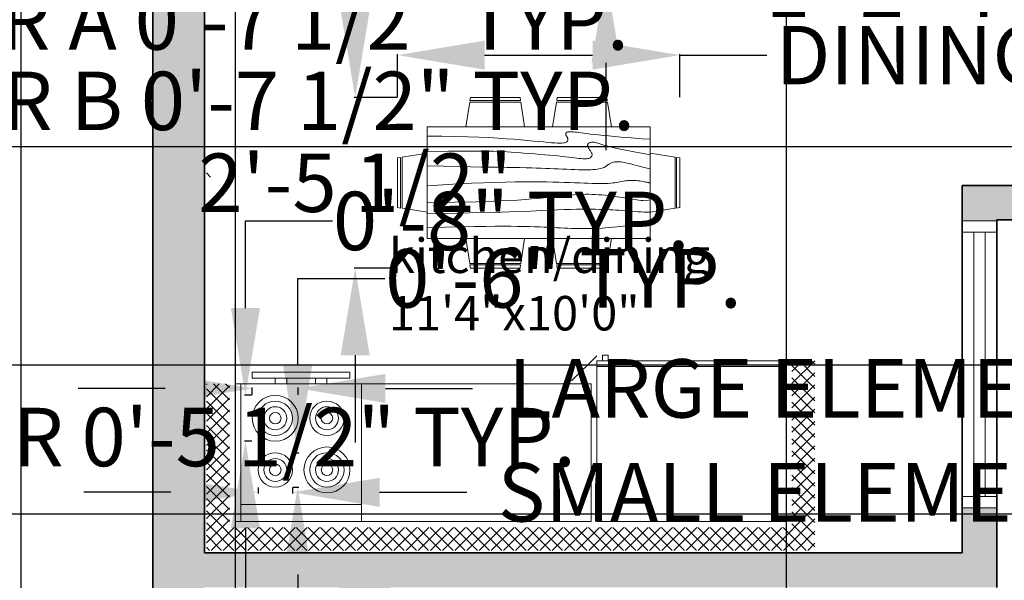
# Model space of a CAD drawing. Units: inches. Extents: x 19 to 15718, y 7 to 930.
# Tile 7 of 11: x 15243 to 15415, y 458 to 556. Entities that reach past the tile are written whole.
import ezdxf

# ---------------------------------------------------------------- set-up
doc = ezdxf.new("R2010")
doc.units = ezdxf.units.IN
doc.header["$MEASUREMENT"] = 0
for name, color, linetype, lineweight in [('A-ANNO-DIMS', 2, 'Continuous', 18), ('A-AREA-IDEN', 7, 'Continuous', 18), ('A-EQPM', 9, 'Continuous', 18), ('A-FLOR-CASE', 8, 'Continuous', 18), ('A-FLOR-CASE-PATT', 252, 'Continuous', 13), ('A-FURN', 8, 'Continuous', 18), ('A-GLAZ', 4, 'Continuous', 18), ('A-WALL', 7, 'Continuous', 35)]:
    doc.layers.add(name, color=color, linetype=linetype, lineweight=lineweight)
doc.layers.add('A-WALL-PATT', color=18, linetype='Continuous', lineweight=13, true_color=0x000000)
doc.styles.add('Annotative', font='arial.ttf')
doc.styles.get("Standard").update_dxf_attribs({"font": 'arial.ttf'})
doc.dimstyles.get("Standard").update_dxf_attribs({"dimtxt": 10.18, "dimasz": 15.18, "dimexe": 0.18, "dimexo": 0.0625, "dimgap": 0.09, "dimtad": 0, "dimtih": 1, "dimtoh": 1, "dimdec": 0, "dimzin": 0, "dimdsep": 46, "dimlunit": 3, "dimtxsty": 'Standard', "dimcen": 0.09, "dimadec": 0, "dimazin": 0, "dimtfac": 1, "dimtdec": 0, "dimtofl": 0, "dimtmove": 0, "dimatfit": 3, "dimfxl": 1, "dimtolj": 1, "dimtzin": 0, "dimarcsym": 0})

# ---------------------------------------------------------------- blocks, each defined once
blk = doc.blocks.new('Dining Set - 36 x 72 in.')
for p, q in [((-22.2343, 26.00059), (-23.4847, 17.99762)), ((-22.2304, 26), (-5.7608, 26)), ((-22, 27.5), (-22.1562, 26.50042)), ((-5.8416, 26.5), (-22.1534, 26.5)), ((-22, 27.5), (-6, 27.5)), ((-5.8437, 26.49966), (-6, 27.5)), ((-4.5152, 17.99762), (-5.7655, 25.99926)), ((5.7657, 26.00059), (4.5153, 17.99762)), ((5.7696, 26), (22.2392, 26)), ((6, 27.5), (5.8438, 26.50042)), ((22.1584, 26.5), (5.8466, 26.5)), ((6, 27.5), (22, 27.5)), ((22.1563, 26.49966), (22, 27.5)), ((23.4848, 17.99762), (22.2345, 25.99926)), ((36, 18), (-36, 18)), ((-36, 18), (-36, -18)), ((36, -18), (36, 18)), ((-45.5, 8), (-44.5004, 8.15617)), ((-45.5, 8), (-45.5, -8)), ((-44.5, -8.15843), (-44.5, 8.15338)), ((-44.0006, 8.23428), (-35.9976, 9.48474)), ((-44, 8.23041), (-44, -8.23915)), ((44.0006, 8.23428), (35.9976, 9.48474)), ((44, 8.23041), (44, -8.23915)), ((44.5, -8.15843), (44.5, 8.15338)), ((45.5, 8), (44.5005, 8.15617)), ((45.5, 8), (45.5, -8)), ((-44.4997, -8.15631), (-45.5, -8)), ((-35.9976, -9.48476), (-43.9993, -8.2345)), ((35.9976, -9.48476), (43.9993, -8.2345)), ((44.4997, -8.15631), (45.5, -8)), ((-36, -18), (36, -18)), ((-22.2343, -26.0006), (-23.4847, -17.99762)), ((-4.5152, -17.99762), (-5.7655, -25.99928)), ((5.7657, -26.0006), (4.5153, -17.99762)), ((23.4848, -17.99762), (22.2345, -25.99928)), ((-22.2304, -26), (-5.7608, -26)), ((-22, -27.5), (-22.1562, -26.50044)), ((-5.8416, -26.5), (-22.1534, -26.5)), ((-22, -27.5), (-6, -27.5)), ((-5.8437, -26.49967), (-6, -27.5)), ((5.7696, -26), (22.2392, -26)), ((6, -27.5), (5.8438, -26.50044)), ((22.1584, -26.5), (5.8466, -26.5)), ((6, -27.5), (22, -27.5)), ((22.1563, -26.49967), (22, -27.5))]:
    blk.add_line(p, q)
for points in [[(-36, 15), (-31.1772, 14.97754), (-26.8079, 14.91406), (-22.8538, 14.81543), (-19.276, 14.6875), (-16.0362, 14.53613), (-13.0957, 14.36718), (-10.4159, 14.18652), (-7.9583, 14), (-5.6904, 13.81315), (-3.6035, 13.63021), (-1.6954, 13.45508), (0.0365, 13.29166), (1.5945, 13.14388), (2.9811, 13.01562), (4.1988, 12.9108), (5.25, 12.83333), (6.1393, 12.78613), (6.8802, 12.76823), (7.4883, 12.77767), (7.9792, 12.8125), (8.3685, 12.87077), (8.6719, 12.95052), (8.9049, 13.0498), (9.0833, 13.16666), (9.2205, 13.29899), (9.3216, 13.44401), (9.3895, 13.59879), (9.4271, 13.76041), (9.4373, 13.92594), (9.4232, 14.09245), (9.3875, 14.257), (9.3333, 14.41666), (9.2638, 14.56917), (9.1836, 14.71484), (9.0975, 14.85465), (9.0104, 14.98958), (8.9272, 15.1206), (8.8529, 15.2487), (8.7922, 15.37483), (8.75, 15.5), (8.7305, 15.62467), (8.7344, 15.74739), (8.7617, 15.86621), (8.8125, 15.97916), (8.8867, 16.08431), (8.9844, 16.17968), (9.1055, 16.26334), (9.25, 16.33333), (9.4189, 16.38802), (9.6172, 16.42708), (9.8506, 16.45052), (10.125, 16.45833), (10.4463, 16.45052), (10.8203, 16.42708), (11.2529, 16.38802), (11.75, 16.33333), (12.3184, 16.26318), (12.9694, 16.17838), (13.7151, 16.07991), (14.5677, 15.96875), (15.5395, 15.84586), (16.6426, 15.71224), (17.8893, 15.56884), (19.2917, 15.41666), (20.859, 15.25667), (22.5879, 15.08984), (24.4721, 14.91715), (26.5052, 14.73958), (28.6809, 14.5581), (30.9929, 14.3737), (33.4347, 14.18733), (36, 14)], [(-36, 10), (-28.9766, 10.14274), (-23.1725, 10.20442), (-18.4241, 10.19775), (-14.5677, 10.13541), (-11.4399, 10.03011), (-8.877, 9.89453), (-6.7154, 9.74137), (-4.7917, 9.58333), (-2.9698, 9.43082), (-1.2246, 9.28515), (0.4415, 9.14534), (2.026, 9.01041), (3.5266, 8.87939), (4.9408, 8.7513), (6.266, 8.62516), (7.5, 8.5), (8.6411, 8.37549), (9.6914, 8.2539), (10.6538, 8.13818), (11.5312, 8.03125), (12.3267, 7.93603), (13.043, 7.85547), (13.6831, 7.79248), (14.25, 7.75), (14.7471, 7.7303), (15.1797, 7.73307), (15.5537, 7.75732), (15.875, 7.80208), (16.1494, 7.86637), (16.3828, 7.94922), (16.5811, 8.04964), (16.75, 8.16666), (16.8944, 8.29915), (17.0143, 8.44531), (17.1089, 8.60319), (17.1771, 8.77083), (17.218, 8.94629), (17.2305, 9.1276), (17.2137, 9.31282), (17.1667, 9.5), (17.0895, 9.6875), (16.987, 9.875), (16.8649, 10.0625), (16.7292, 10.25), (16.5856, 10.4375), (16.4401, 10.625), (16.2985, 10.8125), (16.1667, 11), (16.05, 11.18733), (15.9518, 11.3737), (15.8752, 11.5581), (15.8229, 11.73958), (15.798, 11.91715), (15.8034, 12.08984), (15.842, 12.25667), (15.9167, 12.41666), (16.0295, 12.56836), (16.1784, 12.70833), (16.3605, 12.83268), (16.5729, 12.9375), (16.8127, 13.01888), (17.0768, 13.07291), (17.3625, 13.0957), (17.6667, 13.08333), (17.9894, 13.03312), (18.3418, 12.94726), (18.7382, 12.82918), (19.1927, 12.68229), (19.7195, 12.51001), (20.3327, 12.31575), (21.0465, 12.10294), (21.875, 11.875), (22.8357, 11.63354), (23.959, 11.37304), (25.2786, 11.08618), (26.8282, 10.76562), (28.6414, 10.40405), (30.752, 9.99414), (33.1936, 9.52856), (36, 9)], [(-36, 5.5), (-30.7157, 5.3348), (-26.069, 5.20963), (-21.9946, 5.11767), (-18.4271, 5.05208), (-15.3009, 5.00602), (-12.5508, 4.97265), (-10.1112, 4.94515), (-7.9167, 4.91666), (-5.909, 4.88167), (-4.0586, 4.83984), (-2.3429, 4.79215), (-0.7396, 4.73958), (0.7739, 4.6831), (2.22, 4.6237), (3.6213, 4.56233), (5, 4.5), (6.373, 4.43782), (7.7344, 4.3776), (9.0723, 4.32129), (10.375, 4.27083), (11.6309, 4.22819), (12.8281, 4.19531), (13.9551, 4.17415), (15, 4.16666), (15.954, 4.17448), (16.819, 4.19791), (17.6001, 4.23698), (18.3021, 4.29166), (18.9299, 4.36198), (19.4883, 4.44791), (19.9823, 4.54948), (20.4167, 4.66666), (20.7969, 4.79899), (21.1302, 4.94401), (21.4245, 5.09879), (21.6875, 5.26041), (21.9271, 5.42594), (22.1511, 5.59245), (22.3672, 5.757), (22.5834, 5.91666), (22.8065, 6.06868), (23.0404, 6.21093), (23.2879, 6.34147), (23.5521, 6.45833), (23.8358, 6.55957), (24.142, 6.64323), (24.4735, 6.70735), (24.8334, 6.75), (25.2235, 6.76969), (25.642, 6.76692), (26.0858, 6.74267), (26.5521, 6.69791), (27.0379, 6.63362), (27.5404, 6.55078), (28.0565, 6.45036), (28.5834, 6.33333), (29.1242, 6.19987), (29.7071, 6.04687), (30.3661, 5.87044), (31.1354, 5.66666), (32.0493, 5.43164), (33.142, 5.16146), (34.4475, 4.85221), (36, 4.5)], [(-36, -1), (-30.7915, -0.6591), (-26.0195, -0.38216), (-21.6519, -0.16284), (-17.6563, 0.00521), (-14.0005, 0.12833), (-10.6523, 0.21289), (-7.5796, 0.26522), (-4.75, 0.29166), (-2.134, 0.29793), (0.2878, 0.28711), (2.5317, 0.26163), (4.6146, 0.22396), (6.5529, 0.17651), (8.3633, 0.12174), (10.0623, 0.06209), (11.6667, 0), (13.1899, -0.06201), (14.6341, -0.1211), (15.9982, -0.17432), (17.2813, -0.21875), (18.4823, -0.25147), (19.6003, -0.26953), (20.6343, -0.27002), (21.5834, -0.25), (22.4481, -0.20768), (23.2357, -0.14584), (23.9549, -0.06836), (24.6146, 0.02083), (25.2235, 0.11784), (25.7904, 0.21875), (26.3241, 0.31966), (26.8334, 0.41666), (27.3265, 0.50618), (27.8099, 0.58593), (28.2894, 0.65397), (28.7709, 0.70833), (29.2601, 0.74707), (29.763, 0.76823), (30.2855, 0.76985), (30.8334, 0.75), (31.4088, 0.70784), (31.9994, 0.64713), (32.589, 0.57275), (33.1615, 0.48958), (33.7008, 0.4025), (34.1908, 0.3164), (34.6153, 0.23616), (34.9584, 0.16666), (35.2099, 0.11165), (35.3848, 0.07031), (35.504, 0.04069), (35.5886, 0.02083), (35.6594, 0.00879), (35.7377, 0.0026), (35.8442, 0.00032), (36, 0)], [(-36, -6.5), (-27.1843, -6.31267), (-20.084, -6.1263), (-14.469, -5.9419), (-10.1094, -5.76042), (-6.7752, -5.58285), (-4.2363, -5.41016), (-2.2629, -5.24333), (-0.625, -5.08334), (0.8708, -4.93099), (2.2715, -4.78646), (3.5872, -4.64974), (4.8281, -4.52084), (6.0046, -4.39974), (7.127, -4.28646), (8.2053, -4.18099), (9.25, -4.08334), (10.2705, -3.99382), (11.2734, -3.91407), (12.2647, -3.84603), (13.25, -3.79167), (14.2354, -3.75293), (15.2266, -3.73177), (16.2295, -3.73015), (17.25, -3.75), (18.2912, -3.79248), (19.3451, -3.85547), (20.4009, -3.93604), (21.4479, -4.03125), (22.4754, -4.13819), (23.4727, -4.25391), (24.4289, -4.37549), (25.3334, -4.5), (26.1785, -4.62492), (26.9694, -4.74935), (27.7145, -4.87281), (28.4219, -4.99479), (29.1, -5.11483), (29.7572, -5.23242), (30.4016, -5.34709), (31.0417, -5.45834), (31.6837, -5.56437), (32.3262, -5.65821), (32.9658, -5.73153), (33.599, -5.77604), (34.2224, -5.78345), (34.8327, -5.74545), (35.4264, -5.65373), (36, -5.5)], [(-36, -10), (-26.4022, -9.81299), (-18.4675, -9.62891), (-11.9839, -9.45069), (-6.7396, -9.28125), (-2.5226, -9.12354), (0.8789, -8.98047), (3.6769, -8.85498), (6.0833, -8.75), (8.2767, -8.66765), (10.3021, -8.60677), (12.1712, -8.56543), (13.8958, -8.54167), (15.4876, -8.53353), (16.9583, -8.53907), (18.3197, -8.55632), (19.5834, -8.58334), (20.7616, -8.61841), (21.8685, -8.66081), (22.9188, -8.71004), (23.9271, -8.76563), (24.9081, -8.82707), (25.8763, -8.89388), (26.8465, -8.96558), (27.8334, -9.04167), (28.8474, -9.12118), (29.8828, -9.20117), (30.93, -9.27824), (31.9792, -9.34896), (33.0205, -9.40991), (34.0443, -9.45768), (35.0407, -9.48885), (36, -9.5)], [(-36, -14.5), (-30.0881, -14.33513), (-25.0332, -14.21224), (-20.7312, -14.12647), (-17.0781, -14.07292), (-13.97, -14.04671), (-11.3027, -14.04297), (-8.9724, -14.05681), (-6.875, -14.08334), (-4.9224, -14.11833), (-3.0905, -14.16016), (-1.3709, -14.20785), (0.2448, -14.26042), (1.7647, -14.3169), (3.1973, -14.3763), (4.5507, -14.43767), (5.8333, -14.5), (7.0554, -14.5621), (8.235, -14.62175), (9.3922, -14.67652), (10.5469, -14.72396), (11.7192, -14.76164), (12.929, -14.78711), (14.1965, -14.79794), (15.5417, -14.79167), (16.9933, -14.76424), (18.6152, -14.70508), (20.4804, -14.60197), (22.6615, -14.44271), (25.2312, -14.21509), (28.2624, -13.9069), (31.8277, -13.50594), (36, -13)]]:
    blk.add_lwpolyline(points)
blk = doc.blocks.new('*D17')
at = {"layer": 'A-ANNO-DIMS', "color": 0, "lineweight": -2, "transparency": 16777216}
for p, q in [((15266.62, 830.27), (15243.58, 830.27)), ((15243.76, 815.09), (15243.76, 595.52)), ((15243.76, 365.38), (15243.76, 584.95)), ((15266.62, 350.2), (15243.58, 350.2))]:
    blk.add_line(p, q, dxfattribs=at)
at = {"layer": 'A-ANNO-DIMS', "color": 0, "transparency": 16777216}
for points in [[(15241.23, 815.09), (15246.29, 815.09), (15243.76, 830.27)], [(15241.23, 365.38), (15246.29, 365.38), (15243.76, 350.2)]]:
    blk.add_solid(points, dxfattribs=at)
at = {"layer": 'Defpoints', "color": 0, "transparency": 16777216}
for p in [(15266.68, 830.27), (15243.76, 350.2), (15266.68, 350.2)]:
    blk.add_point(p, dxfattribs=at)
at = {"layer": 'A-ANNO-DIMS', "color": 0, "transparency": 16777216, "insert": (15243.76, 590.24), "char_height": 10.18, "attachment_point": 5}
blk.add_mtext("\\A1;40'", dxfattribs=at)
blk = doc.blocks.new('HOB-ELECTRIC-6IN')
for radius in [3, 2, 1]:
    blk.add_circle((3, 3), radius)
blk = doc.blocks.new('HOB-ELECTRIC-8IN')
for radius in [4, 3, 2, 1]:
    blk.add_circle((4, 4), radius)
blk = doc.blocks.new('*D40')
at = {"layer": 'A-ANNO-DIMS', "color": 0, "lineweight": -2, "transparency": 16777216}
for p, q in [((15117.25, 555.92), (15102.07, 555.92)), ((15132.43, 556.96), (15132.43, 555.74)), ((15139.78, 556.96), (15139.78, 555.74)), ((15154.96, 555.92), (15170.14, 555.92))]:
    blk.add_line(p, q, dxfattribs=at)
at = {"layer": 'A-ANNO-DIMS', "color": 0, "transparency": 16777216}
for points in [[(15117.25, 558.45), (15117.25, 553.39), (15132.43, 555.92)], [(15154.96, 558.45), (15154.96, 553.39), (15139.78, 555.92)]]:
    blk.add_solid(points, dxfattribs=at)
at = {"layer": 'Defpoints', "color": 0, "transparency": 16777216}
for p in [(15132.43, 557.02), (15139.78, 557.02), (15139.78, 555.92)]:
    blk.add_point(p, dxfattribs=at)
at = {"layer": 'A-ANNO-DIMS', "color": 0, "transparency": 16777216, "insert": (15262.49, 555.92), "char_height": 10.18, "attachment_point": 5}
blk.add_mtext('\\A1;SIDE CHAIR A 0\'-7 1/2" TYP.', dxfattribs=at)
blk = doc.blocks.new('*D42')
at = {"layer": 'A-ANNO-DIMS', "color": 0, "lineweight": -2, "transparency": 16777216}
for p, q in [((15133.17, 540.88), (15133.17, 542.1)), ((15140.52, 540.88), (15140.52, 542.1)), ((15117.99, 541.92), (15102.81, 541.92)), ((15155.7, 541.92), (15170.88, 541.92))]:
    blk.add_line(p, q, dxfattribs=at)
at = {"layer": 'A-ANNO-DIMS', "color": 0, "transparency": 16777216}
for points in [[(15117.99, 544.45), (15117.99, 539.39), (15133.17, 541.92)], [(15155.7, 544.45), (15155.7, 539.39), (15140.52, 541.92)]]:
    blk.add_solid(points, dxfattribs=at)
at = {"layer": 'Defpoints', "color": 0, "transparency": 16777216}
for p in [(15133.17, 540.82), (15140.52, 541.92), (15140.52, 540.82)]:
    blk.add_point(p, dxfattribs=at)
at = {"layer": 'A-ANNO-DIMS', "color": 0, "transparency": 16777216, "insert": (15263.22, 541.92), "char_height": 10.18, "attachment_point": 5}
blk.add_mtext('\\A1;SIDE CHAIR B 0\'-7 1/2" TYP.', dxfattribs=at)
blk = doc.blocks.new('*D60')
at = {"layer": 'A-ANNO-DIMS', "color": 0, "lineweight": -2, "transparency": 16777216}
for p, q in [((15125.78, 484.16), (15125.78, 483.21)), ((15131.32, 484.16), (15131.32, 483.21)), ((15110.6, 483.39), (15095.42, 483.39)), ((15146.5, 483.39), (15161.68, 483.39))]:
    blk.add_line(p, q, dxfattribs=at)
at = {"layer": 'A-ANNO-DIMS', "color": 0, "transparency": 16777216}
for points in [[(15110.6, 485.92), (15110.6, 480.86), (15125.78, 483.39)], [(15146.5, 485.92), (15146.5, 480.86), (15131.32, 483.39)]]:
    blk.add_solid(points, dxfattribs=at)
at = {"layer": 'Defpoints', "color": 0, "transparency": 16777216}
for p in [(15125.78, 484.23), (15131.32, 484.23), (15131.32, 483.39)]:
    blk.add_point(p, dxfattribs=at)
at = {"layer": 'A-ANNO-DIMS', "color": 0, "transparency": 16777216, "insert": (15253.56, 483.39), "char_height": 10.18, "attachment_point": 5}
blk.add_mtext('\\A1;GAS BURNER 0\'-5 1/2" TYP.', dxfattribs=at)
blk = doc.blocks.new('*D62')
at = {"layer": 'A-ANNO-DIMS', "color": 0, "lineweight": -2, "transparency": 16777216}
for p, q in [((15269.83, 473.76), (15254.65, 473.76)), ((15285.01, 474.6), (15285.01, 473.58)), ((15291.01, 474.6), (15291.01, 473.58)), ((15306.19, 473.76), (15321.37, 473.76))]:
    blk.add_line(p, q, dxfattribs=at)
at = {"layer": 'A-ANNO-DIMS', "color": 0, "transparency": 16777216}
for points in [[(15269.83, 476.29), (15269.83, 471.23), (15285.01, 473.76)], [(15306.19, 476.29), (15306.19, 471.23), (15291.01, 473.76)]]:
    blk.add_solid(points, dxfattribs=at)
at = {"layer": 'Defpoints', "color": 0, "transparency": 16777216}
for p in [(15285.01, 474.66), (15291.01, 474.66), (15291.01, 473.76)]:
    blk.add_point(p, dxfattribs=at)
at = {"layer": 'A-ANNO-DIMS', "color": 0, "transparency": 16777216, "insert": (15413.32, 473.76), "char_height": 10.18, "attachment_point": 5}
blk.add_mtext('\\A1;SMALL ELEMENT 0\'-6" TYP.', dxfattribs=at)
blk = doc.blocks.new('*D63')
at = {"layer": 'A-ANNO-DIMS', "color": 0, "lineweight": -2, "transparency": 16777216}
for p, q in [((15291.91, 495.84), (15291.91, 511.02)), ((15291.91, 511.02), (15307.09, 511.02)), ((15291.07, 480.66), (15292.09, 480.66)), ((15291.07, 474.66), (15292.09, 474.66)), ((15291.91, 459.48), (15291.91, 444.3))]:
    blk.add_line(p, q, dxfattribs=at)
at = {"layer": 'A-ANNO-DIMS', "color": 0, "transparency": 16777216}
for points in [[(15289.38, 495.84), (15294.44, 495.84), (15291.91, 480.66)], [(15289.38, 459.48), (15294.44, 459.48), (15291.91, 474.66)]]:
    blk.add_solid(points, dxfattribs=at)
at = {"layer": 'Defpoints', "color": 0, "transparency": 16777216}
for p in [(15291.01, 480.66), (15291.91, 480.66), (15291.01, 474.66)]:
    blk.add_point(p, dxfattribs=at)
at = {"layer": 'A-ANNO-DIMS', "color": 0, "transparency": 16777216, "insert": (15338.21, 511.02), "char_height": 10.18, "attachment_point": 5}
blk.add_mtext('\\A1;0\'-6" TYP.', dxfattribs=at)
blk = doc.blocks.new('*D64')
at = {"layer": 'A-ANNO-DIMS', "color": 0, "lineweight": -2, "transparency": 16777216}
for p, q in [((15268.83, 491.86), (15253.65, 491.86)), ((15284.01, 490.72), (15284.01, 492.04)), ((15292.01, 490.72), (15292.01, 492.04)), ((15307.19, 491.86), (15322.37, 491.86))]:
    blk.add_line(p, q, dxfattribs=at)
at = {"layer": 'A-ANNO-DIMS', "color": 0, "transparency": 16777216}
for points in [[(15268.83, 494.39), (15268.83, 489.33), (15284.01, 491.86)], [(15307.19, 494.39), (15307.19, 489.33), (15292.01, 491.86)]]:
    blk.add_solid(points, dxfattribs=at)
at = {"layer": 'Defpoints', "color": 0, "transparency": 16777216}
for p in [(15284.01, 490.66), (15292.01, 491.86), (15292.01, 490.66)]:
    blk.add_point(p, dxfattribs=at)
at = {"layer": 'A-ANNO-DIMS', "color": 0, "transparency": 16777216, "insert": (15414.9, 491.86), "char_height": 10.18, "attachment_point": 5}
blk.add_mtext('\\A1;LARGE ELEMENT 0\'-8" TYP.', dxfattribs=at)
blk = doc.blocks.new('*D65')
at = {"layer": 'A-ANNO-DIMS', "color": 0, "lineweight": -2, "transparency": 16777216}
for p, q in [((15282.81, 505.84), (15282.81, 521.02)), ((15282.81, 521.02), (15297.99, 521.02)), ((15283.95, 490.66), (15282.63, 490.66)), ((15283.95, 482.66), (15282.63, 482.66)), ((15282.81, 467.48), (15282.81, 452.3))]:
    blk.add_line(p, q, dxfattribs=at)
at = {"layer": 'A-ANNO-DIMS', "color": 0, "transparency": 16777216}
for points in [[(15280.28, 505.84), (15285.34, 505.84), (15282.81, 490.66)], [(15280.28, 467.48), (15285.34, 467.48), (15282.81, 482.66)]]:
    blk.add_solid(points, dxfattribs=at)
at = {"layer": 'Defpoints', "color": 0, "transparency": 16777216}
for p in [(15282.81, 490.66), (15284.01, 490.66), (15284.01, 482.66)]:
    blk.add_point(p, dxfattribs=at)
at = {"layer": 'A-ANNO-DIMS', "color": 0, "transparency": 16777216, "insert": (15329.11, 521.02), "char_height": 10.18, "attachment_point": 5}
blk.add_mtext('\\A1;0\'-8" TYP.', dxfattribs=at)
blk = doc.blocks.new('*D66')
at = {"layer": 'A-ANNO-DIMS', "color": 0, "lineweight": -2, "transparency": 16777216}
for p, q in [((15345.61, 592.88), (15345.61, 608.06)), ((15343.57, 577.7), (15345.79, 577.7)), ((15343.57, 563.7), (15345.79, 563.7)), ((15345.61, 548.52), (15345.61, 533.34))]:
    blk.add_line(p, q, dxfattribs=at)
at = {"layer": 'A-ANNO-DIMS', "color": 0, "transparency": 16777216}
for points in [[(15343.08, 592.88), (15348.14, 592.88), (15345.61, 577.7)], [(15343.08, 548.52), (15348.14, 548.52), (15345.61, 563.7)]]:
    blk.add_solid(points, dxfattribs=at)
at = {"layer": 'Defpoints', "color": 0, "transparency": 16777216}
for p in [(15343.51, 577.7), (15345.61, 577.7), (15343.51, 563.7)]:
    blk.add_point(p, dxfattribs=at)
at = {"layer": 'A-ANNO-DIMS', "color": 0, "transparency": 16777216, "insert": (15345.61, 570.7), "char_height": 10.18, "attachment_point": 5}
blk.add_mtext('\\A1;SINK BOWL 1\'-2" TYP.', dxfattribs=at)
blk = doc.blocks.new('*D67')
at = {"layer": 'A-ANNO-DIMS', "color": 0, "lineweight": -2, "transparency": 16777216}
for p, q in [((15329.76, 563.64), (15329.76, 561.42)), ((15343.51, 563.64), (15343.51, 561.42)), ((15314.58, 561.6), (15299.4, 561.6)), ((15358.69, 561.6), (15373.87, 561.6))]:
    blk.add_line(p, q, dxfattribs=at)
at = {"layer": 'A-ANNO-DIMS', "color": 0, "transparency": 16777216}
for points in [[(15314.58, 564.13), (15314.58, 559.07), (15329.76, 561.6)], [(15358.69, 564.13), (15358.69, 559.07), (15343.51, 561.6)]]:
    blk.add_solid(points, dxfattribs=at)
at = {"layer": 'Defpoints', "color": 0, "transparency": 16777216}
for p in [(15329.76, 563.7), (15343.51, 563.7), (15343.51, 561.6)]:
    blk.add_point(p, dxfattribs=at)
at = {"layer": 'A-ANNO-DIMS', "color": 0, "transparency": 16777216, "insert": (15404.51, 561.6), "char_height": 10.18, "attachment_point": 5}
blk.add_mtext('\\A1;1\'-2" TYP.', dxfattribs=at)
blk = doc.blocks.new('*D68')
at = {"layer": 'A-ANNO-DIMS', "color": 0, "lineweight": -2, "transparency": 16777216}
for p, q in [((15309.3, 542.58), (15309.3, 550.07)), ((15324.48, 549.89), (15343.27, 549.89)), ((15358.45, 542.58), (15358.45, 550.07)), ((15358.45, 549.89), (15373.63, 549.89))]:
    blk.add_line(p, q, dxfattribs=at)
at = {"layer": 'A-ANNO-DIMS', "color": 0, "transparency": 16777216}
for points in [[(15324.48, 552.42), (15324.48, 547.36), (15309.3, 549.89)], [(15343.27, 552.42), (15343.27, 547.36), (15358.45, 549.89)]]:
    blk.add_solid(points, dxfattribs=at)
at = {"layer": 'Defpoints', "color": 0, "transparency": 16777216}
for p in [(15358.45, 549.89), (15309.3, 542.52), (15358.45, 542.52)]:
    blk.add_point(p, dxfattribs=at)
at = {"layer": 'A-ANNO-DIMS', "color": 0, "transparency": 16777216, "insert": (15429.66, 549.89), "char_height": 10.18, "attachment_point": 5}
blk.add_mtext('\\A1;DINING SET 4\'-1"', dxfattribs=at)
blk = doc.blocks.new('*D69')
at = {"layer": 'A-ANNO-DIMS', "color": 0, "lineweight": -2, "transparency": 16777216}
for p, q in [((15301.93, 557.7), (15301.93, 572.88)), ((15309.24, 542.52), (15301.75, 542.52)), ((15309.24, 512.82), (15301.75, 512.82)), ((15301.93, 497.64), (15301.93, 482.46))]:
    blk.add_line(p, q, dxfattribs=at)
at = {"layer": 'A-ANNO-DIMS', "color": 0, "transparency": 16777216}
for points in [[(15299.4, 557.7), (15304.46, 557.7), (15301.93, 542.52)], [(15299.4, 497.64), (15304.46, 497.64), (15301.93, 512.82)]]:
    blk.add_solid(points, dxfattribs=at)
at = {"layer": 'Defpoints', "color": 0, "transparency": 16777216}
for p in [(15301.93, 542.52), (15309.3, 542.52), (15309.3, 512.82)]:
    blk.add_point(p, dxfattribs=at)
at = {"layer": 'A-ANNO-DIMS', "color": 0, "transparency": 16777216, "insert": (15301.93, 527.67), "char_height": 10.18, "attachment_point": 5}
blk.add_mtext('\\A1;2\'-5 1/2"', dxfattribs=at)
blk = doc.blocks.new('*D79')
at = {"layer": 'A-ANNO-DIMS', "color": 0, "lineweight": -2, "transparency": 16777216}
for p, q in [((15602.03, 534), (15602.03, 549.18)), ((15602.03, 549.18), (15617.21, 549.18)), ((15082.89, 534), (15602.21, 534)), ((15602.03, 511.14), (15602.03, 518.82)), ((15082.89, 495.96), (15602.21, 495.96))]:
    blk.add_line(p, q, dxfattribs=at)
at = {"layer": 'A-ANNO-DIMS', "color": 0, "transparency": 16777216}
for points in [[(15599.5, 518.82), (15604.56, 518.82), (15602.03, 534)], [(15599.5, 511.14), (15604.56, 511.14), (15602.03, 495.96)]]:
    blk.add_solid(points, dxfattribs=at)
at = {"layer": 'Defpoints', "color": 0, "transparency": 16777216}
for p in [(15082.83, 534), (15602.03, 534), (15082.83, 495.96)]:
    blk.add_point(p, dxfattribs=at)
at = {"layer": 'A-ANNO-DIMS', "color": 0, "transparency": 16777216, "insert": (15630.83, 549.18), "char_height": 10.18, "attachment_point": 5}
blk.add_mtext('\\A1;3\'-2"', dxfattribs=at)
blk = doc.blocks.new('*D80')
at = {"layer": 'A-ANNO-DIMS', "color": 0, "lineweight": -2, "transparency": 16777216}
for p, q in [((15602.030581, 511.142303), (15602.030581, 526.322303)), ((15181.899116, 495.962303), (15602.210581, 495.962303)), ((15181.899116, 469.995573), (15602.210581, 469.995573)), ((15602.030581, 454.815573), (15602.030581, 439.635573))]:
    blk.add_line(p, q, dxfattribs=at)
at = {"layer": 'A-ANNO-DIMS', "color": 0, "transparency": 16777216}
for points in [[(15599.500581, 511.142303), (15604.560581, 511.142303), (15602.030581, 495.962303)], [(15599.500581, 454.815573), (15604.560581, 454.815573), (15602.030581, 469.995573)]]:
    blk.add_solid(points, dxfattribs=at)
at = {"layer": 'Defpoints', "color": 0, "transparency": 16777216}
for p in [(15181.836616, 495.962303), (15602.030581, 495.962303), (15181.836616, 469.995573)]:
    blk.add_point(p, dxfattribs=at)
at = {"layer": 'A-ANNO-DIMS', "color": 0, "transparency": 16777216, "insert": (15602.030581, 482.978938), "char_height": 10.18, "attachment_point": 5}
blk.add_mtext('\\A1;2\'-2"', dxfattribs=at)
blk = doc.blocks.new('*D81')
at = {"layer": 'A-ANNO-DIMS', "color": 0, "lineweight": -2, "transparency": 16777216}
for p, q in [((15281.01, 559.14), (15281.01, 314.67)), ((15377.01, 559.14), (15377.01, 314.67)), ((15296.19, 314.85), (15315.38, 314.85)), ((15361.83, 314.85), (15342.64, 314.85))]:
    blk.add_line(p, q, dxfattribs=at)
at = {"layer": 'A-ANNO-DIMS', "color": 0, "transparency": 16777216}
for points in [[(15296.19, 317.38), (15296.19, 312.32), (15281.01, 314.85)], [(15361.83, 317.38), (15361.83, 312.32), (15377.01, 314.85)]]:
    blk.add_solid(points, dxfattribs=at)
at = {"layer": 'Defpoints', "color": 0, "transparency": 16777216}
for p in [(15281.01, 559.2), (15377.01, 559.2), (15377.01, 314.85)]:
    blk.add_point(p, dxfattribs=at)
at = {"layer": 'A-ANNO-DIMS', "color": 0, "transparency": 16777216, "insert": (15329.01, 314.85), "char_height": 10.18, "attachment_point": 5}
blk.add_mtext('\\A1;8\'-0"', dxfattribs=at)
blk = doc.blocks.new('*D82')
at = {"layer": 'A-ANNO-DIMS', "color": 0, "lineweight": -2, "transparency": 16777216}
for p, q in [((15602.030581, 598.383955), (15602.030581, 613.563955)), ((15377.073779, 583.203955), (15602.210581, 583.203955)), ((15377.073779, 559.203955), (15602.210581, 559.203955)), ((15602.030581, 544.023955), (15602.030581, 528.843955))]:
    blk.add_line(p, q, dxfattribs=at)
at = {"layer": 'A-ANNO-DIMS', "color": 0, "transparency": 16777216}
for points in [[(15599.500581, 598.383955), (15604.560581, 598.383955), (15602.030581, 583.203955)], [(15599.500581, 544.023955), (15604.560581, 544.023955), (15602.030581, 559.203955)]]:
    blk.add_solid(points, dxfattribs=at)
at = {"layer": 'Defpoints', "color": 0, "transparency": 16777216}
for p in [(15377.011279, 583.203955), (15602.030581, 583.203955), (15377.011279, 559.203955)]:
    blk.add_point(p, dxfattribs=at)
at = {"layer": 'A-ANNO-DIMS', "color": 0, "transparency": 16777216, "insert": (15602.030581, 571.203955), "char_height": 10.18, "attachment_point": 5}
blk.add_mtext('\\A1;2\'-0"', dxfattribs=at)

msp = doc.modelspace()

# ---------------------------------------------------------------- hatches: boundary and pattern name
at = {"layer": 'A-FLOR-CASE-PATT'}
h = msp.add_hatch(dxfattribs=at)
h.set_pattern_fill('ANSI37', color=256, scale=12, style=0)
h.paths.add_polyline_path([(15276.01, 463.66), (15382.01, 463.66), (15382.01, 496.66), (15378.01, 496.66), (15378.01, 467.66), (15280.01, 467.66), (15280.01, 492.66), (15276.01, 492.66)])
at = {"layer": 'A-WALL-PATT'}
h = msp.add_hatch(color=256, dxfattribs=at)
h.dxf.hatch_style = 1
h.paths.add_polyline_path([(15190.84, 837), (14890.84, 837), (14890.84, 357), (14899.84, 357), (14899.84, 366), (14899.84, 528), (14904.84, 528), (14904.84, 534), (14899.84, 534), (14899.84, 698), (15004.84, 698), (15004.84, 701, -0.014283), (15004.84, 703), (15004.84, 704), (14899.84, 704), (14899.84, 828), (14987.26, 828), (15043.84, 828), (15049.84, 828), (15075.84, 828), (15081.84, 828), (15181.84, 828), (15181.84, 780), (15114.84, 780), (15114.84, 779, -0.017236), (15114.84, 777), (15114.84, 774), (15181.84, 774), (15181.84, 654), (15181.84, 648), (15181.84, 596), (15190.84, 596)])
h.paths.add_polyline_path([(15190.84, 590), (15181.84, 590), (15181.84, 470), (15181.84, 464), (15181.84, 361.43), (14991.9, 361.43), (14991.5, 357), (15190.84, 357)], flags=0)
h.paths.add_polyline_path([(15152.29, 608), (15146.29, 608), (15146.29, 596), (15049.84, 596), (15049.84, 590), (15152.29, 590)], flags=17)
h.paths.add_polyline_path([(15049.84, 615), (15048.84, 615, -0.017236), (15046.84, 615), (15043.84, 615), (15043.84, 596), (15049.84, 596)], flags=17)
edge = h.paths.add_edge_path(flags=17)
edge.add_line((15152.29, 654), (15049.84, 654))
edge.add_line((15049.84, 654), (15043.84, 654))
edge.add_line((15043.84, 654), (15043.84, 648))
edge.add_line((15043.84, 648), (15049.84, 648))
edge.add_line((15049.84, 648), (15075.84, 648))
edge.add_line((15075.84, 648), (15081.84, 648))
edge.add_line((15081.84, 648), (15117.26, 648))
edge.add_spline(control_points=[(15117.26, 648), (15117.59, 648.02), (15117.94, 648.03), (15118.71, 648.04), (15119.15, 648.02), (15119.59, 648)], knot_values=[1.499122, 1.499122, 1.499122, 1.499122, 1.618335, 1.618335, 1.770388, 1.770388, 1.770388, 1.770388], degree=3, periodic=0)
edge.add_spline(control_points=[(15127.99, 642.93), (15128, 643.28), (15127.95, 643.62), (15127.73, 644.26), (15127.57, 644.57), (15127.16, 645.13), (15126.92, 645.39), (15126.04, 646.16), (15125.28, 646.6), (15123.53, 647.31), (15122.55, 647.59), (15120.88, 647.88), (15120.24, 647.95), (15119.59, 648)], knot_values=[0, 0, 0, 0, 0.172075, 0.172075, 0.344149, 0.344149, 0.516224, 0.516224, 0.894541, 0.894541, 1.272858, 1.272858, 1.499122, 1.499122, 1.499122, 1.499122], degree=3, periodic=0)
edge.add_line((15119.59, 648), (15146.29, 648))
edge.add_line((15146.29, 648), (15146.29, 636))
edge.add_line((15146.29, 636), (15152.29, 636))
edge.add_line((15152.29, 636), (15152.29, 654))
h.paths.add_polyline_path([(15132.35, 430.4), (15123.35, 430.4), (15123.35, 396.8), (15027.77, 396.8), (15027.77, 387.8), (15132.35, 387.8)], flags=17)
h.paths.add_polyline_path([(15132.35, 464), (15123.35, 464), (15123.35, 430.4), (15132.35, 430.4)], flags=17)
h.paths.add_polyline_path([(15275.68, 583.59), (15276.07, 583.2), (15276.65, 583.2), (15280.6, 587.16), (15278.55, 589.2), (15275.68, 589.2), (15275.68, 601.2), (15266.68, 601.2), (15266.68, 350.2), (15275.68, 350.2), (15275.68, 359.2), (15275.68, 457.2), (15413.68, 457.2), (15413.68, 471.04), (15407.68, 471.04), (15407.68, 463.2), (15275.68, 463.2)])
h = msp.add_hatch(color=256, dxfattribs=at)
h.dxf.hatch_style = 1
h.paths.add_polyline_path([(15566.68, 830.2), (15266.68, 830.2), (15266.68, 629.2), (15275.68, 629.2), (15275.68, 641.2), (15301.68, 641.2), (15301.68, 589.2), (15275.68, 589.2), (15275.68, 601.2), (15266.68, 601.2), (15266.68, 350.2), (15275.68, 350.2), (15275.68, 359.2), (15275.68, 457.2), (15413.68, 457.2), (15413.68, 471.04), (15407.68, 471.04), (15407.68, 463.2), (15275.68, 463.2), (15275.68, 583.59), (15276.07, 583.2), (15276.65, 583.2), (15277.42, 583.97), (15276.36, 585.03), (15279.54, 588.22), (15280.6, 587.16), (15281.66, 588.22), (15282.72, 587.16), (15283.78, 588.22), (15284.85, 587.16), (15285.91, 588.22), (15286.97, 587.16), (15288.03, 588.22), (15289.09, 587.16), (15290.15, 588.22), (15291.21, 587.16), (15292.27, 588.22), (15293.33, 587.16), (15294.39, 588.22), (15295.45, 587.16), (15296.51, 588.22), (15297.57, 587.16), (15298.63, 588.22), (15299.69, 587.16), (15300.76, 588.22), (15301.82, 587.16), (15302.88, 588.22), (15303.94, 587.16), (15305, 588.22), (15306.06, 587.16), (15307.68, 588.78), (15307.68, 641.2), (15407.68, 641.2), (15413.68, 641.2), (15413.68, 647.2), (15407.68, 647.2), (15275.68, 647.2), (15275.68, 767.2), (15336.68, 767.2), (15336.68, 773.2), (15275.68, 773.2), (15275.68, 821.2), (15375.68, 821.2), (15381.68, 821.2), (15407.68, 821.2), (15413.68, 821.2), (15557.68, 821.2), (15557.68, 697.2), (15452.68, 697.2), (15452.68, 696.2, -0.014283), (15452.68, 694.2), (15452.68, 691.2), (15557.68, 691.2), (15557.68, 527.2), (15557.68, 521.2), (15557.68, 359.2), (15557.68, 350.2), (15566.68, 350.2)])
h.paths.add_polyline_path([(15416.63, 527.2), (15413.68, 527.2), (15407.68, 527.2), (15407.68, 521.04), (15413.68, 521.04), (15413.68, 521.2), (15416.63, 521.2)], flags=17)
h.paths.add_polyline_path([(15432.13, 393.97), (15308.13, 393.97), (15308.13, 425.59), (15299.13, 425.59), (15299.13, 384.97), (15432.13, 384.97)], flags=17)
h.paths.add_polyline_path([(15308.13, 457.2), (15299.13, 457.2), (15299.13, 425.59), (15308.13, 425.59)], flags=17)
h.paths.add_polyline_path([(15425.57, 359.2), (15275.68, 359.2), (15275.68, 350.2), (15425.57, 350.2)], flags=17)
h.paths.add_polyline_path([(15413.68, 797.2), (15407.68, 797.2), (15407.68, 773.2), (15381.68, 773.2), (15381.68, 797.2), (15375.68, 797.2), (15375.68, 773.2), (15375.68, 767.2), (15407.68, 767.2), (15407.68, 686.2), (15408.68, 686.2, -0.014283), (15410.68, 686.2), (15413.68, 686.2), (15413.68, 691.2), (15413.68, 697.2)], flags=17)
h.paths.add_polyline_path([(15413.68, 608.2), (15410.68, 608.2, -0.017236), (15408.68, 608.2), (15407.68, 608.2), (15407.68, 589.2), (15388.16, 589.2, -0.313626), (15386.75, 588.23), (15381.37, 588.23), (15380.3, 587.16), (15381.37, 586.1), (15380.3, 585.03), (15382.14, 583.2), (15407.68, 583.2), (15413.68, 583.2)], flags=17)

# ---------------------------------------------------------------- linework, layer by layer
at = {"layer": 'A-EQPM'}
for p, q in [((15345.01, 497.66), (15346.01, 497.66)), ((15345.01, 496.66), (15345.01, 497.66)), ((15346.01, 497.66), (15346.01, 496.66)), ((15377.01, 495.66), (15344.01, 495.66)), ((15288.01, 492.66), (15288.01, 493.66)), ((15290.01, 493.66), (15290.01, 492.66)), ((15295.01, 493.66), (15295.01, 492.66)), ((15297.01, 492.66), (15297.01, 493.66)), ((15303.01, 471.66), (15282.01, 471.66))]:
    msp.add_line(p, q, dxfattribs=at)
for points in [[(15377.01, 496.66), (15377.01, 468.66), (15344.01, 468.66), (15344.01, 496.66)], [(15301.01, 494.66), (15301.01, 493.66), (15284.01, 493.66), (15284.01, 494.66)], [(15303.01, 492.66), (15303.01, 468.66), (15282.01, 468.66), (15282.01, 492.66)]]:
    msp.add_lwpolyline(points, close=True, dxfattribs=at)
at = {"layer": 'A-FLOR-CASE'}
for p, q in [((15281.01, 492.66), (15343.01, 492.66)), ((15281.01, 468.66), (15281.01, 492.66)), ((15343.01, 492.66), (15343.01, 468.66)), ((15343.01, 468.66), (15281.01, 468.66))]:
    msp.add_line(p, q, dxfattribs=at)
at = {"layer": 'A-FLOR-CASE-PATT'}
for p, q in [((15276.01, 529.38), (15276.73, 528.66)), ((15343.99, 497.55), (15339.6, 493.16))]:
    msp.add_line(p, q, dxfattribs=at)
at = {"layer": 'A-GLAZ'}
for p, q in [((15413.68, 521.04), (15407.68, 521.04)), ((15413.68, 519.04), (15407.68, 519.04)), ((15409.68, 519.04), (15409.68, 473.04)), ((15411.68, 519.04), (15411.68, 473.04)), ((15413.68, 473.04), (15407.68, 473.04)), ((15413.68, 471.04), (15407.68, 471.04))]:
    msp.add_line(p, q, dxfattribs=at)
at = {"layer": 'A-WALL'}
for p, q in [((15266.68, 350.2), (15266.68, 830.2)), ((15275.68, 463.2), (15275.68, 583.2)), ((15407.68, 527.2), (15407.68, 463.2)), ((15413.68, 527.2), (15407.68, 527.2)), ((15413.68, 527.2), (15451.65, 527.2)), ((15413.68, 521.2), (15449.68, 521.2)), ((15413.68, 521.2), (15413.68, 457.2)), ((15275.68, 463.2), (15407.68, 463.2))]:
    msp.add_line(p, q, dxfattribs=at)

# ---------------------------------------------------------------- block references
at = {"layer": 'A-EQPM'}
for name, p in [('HOB-ELECTRIC-8IN', (15284.01, 482.66)), ('HOB-ELECTRIC-6IN', (15285.01, 474.66))]:
    msp.add_blockref(name, p, dxfattribs=at)
for name, p, rotation in [('HOB-ELECTRIC-6IN', (15293.96, 483.71), 359.1052631019651), ('HOB-ELECTRIC-8IN', (15292.95, 481.6), 270.8951737102111)]:
    msp.add_blockref(name, p, dxfattribs=dict(at, rotation=rotation))
at = {"layer": 'A-FURN', "xscale": 0.5400703499232784, "yscale": 0.5400703499232784, "zscale": 0.5400703499232784}
msp.add_blockref('Dining Set - 36 x 72 in.', (15333.88, 527.67), dxfattribs=at)

# ---------------------------------------------------------------- texts
at = {"layer": 'A-AREA-IDEN', "insert": (15307.81, 517.95), "char_height": 6, "width": 68.1983, "attachment_point": 1, "style": 'Annotative'}
msp.add_mtext('kitchen/dining\\P11\'4"x10\'0"', dxfattribs=at)

# ---------------------------------------------------------------- dimensions: what is measured, and where the dimension line sits
at = {"layer": 'A-ANNO-DIMS'}
for base, p1, p2, override, picture, middle in [((15243.76, 350.2), (15266.68, 830.27), (15266.68, 350.2), {"dimclrd": 0, "dimclre": 0, "dimclrt": 0}, '*D17', (15243.76, 590.24)), ((15602.03, 583.2), (15377.01, 559.2), (15377.01, 583.2), {"dimdec": 1, "dimlfac": 1, "dimrnd": 0, "dimzin": 1, "dimdsep": 46, "dimlunit": 4, "dimfrac": 2}, '*D82', (15602.03, 571.2)), ((15301.93, 542.52), (15309.3, 512.82), (15309.3, 542.52), {"dimdec": 1, "dimlfac": 1, "dimrnd": 0, "dimzin": 1, "dimdsep": 46, "dimlunit": 4, "dimfrac": 2}, '*D69', (15301.93, 527.67)), ((15602.03, 534), (15082.83, 495.96), (15082.83, 534), {"dimdec": 1, "dimlfac": 1, "dimrnd": 0, "dimzin": 1, "dimdsep": 46, "dimlunit": 4, "dimfrac": 2}, '*D79', (15630.83, 549.18)), ((15602.03, 495.96), (15181.84, 470), (15181.84, 495.96), {"dimdec": 1, "dimlfac": 1, "dimrnd": 0, "dimzin": 1, "dimdsep": 46, "dimlunit": 4, "dimfrac": 2}, '*D80', (15602.03, 482.98))]:
    dim = msp.add_linear_dim(base=base, p1=p1, p2=p2, angle=90, dimstyle='Standard', override=override, dxfattribs=at)
    dim.commit()
    dim.dimension.update_dxf_attribs({"geometry": picture, "text_midpoint": middle})
for base, p1, p2, text, picture, middle in [((15345.61, 577.7), (15343.51, 563.7), (15343.51, 577.7), 'SINK BOWL <> TYP.', '*D66', (15345.61, 570.7)), ((15282.81, 490.66), (15284.01, 482.66), (15284.01, 490.66), '<> TYP.', '*D65', (15329.11, 521.02)), ((15291.91, 480.66), (15291.01, 474.66), (15291.01, 480.66), '<> TYP.', '*D63', (15338.21, 511.02))]:
    dim = msp.add_linear_dim(base=base, p1=p1, p2=p2, angle=90, text=text, dimstyle='Standard', override={"dimdec": 1, "dimlfac": 1, "dimrnd": 0, "dimzin": 1, "dimdsep": 46, "dimlunit": 4, "dimfrac": 2}, dxfattribs=at)
    dim.commit()
    dim.dimension.update_dxf_attribs({"geometry": picture, "text_midpoint": middle})
for base, p1, p2, text, picture, middle in [((15139.7848, 555.9195), (15132.4322, 557.0224), (15139.7848, 557.0224), 'SIDE CHAIR A <> TYP.', '*D40', (15262.4867, 555.9195)), ((15140.519, 541.924), (15133.1663, 540.8211), (15140.519, 540.8211), 'SIDE CHAIR B <> TYP.', '*D42', (15263.2209, 541.924)), ((15343.51127927, 561.60395495), (15329.76127927, 563.70395495), (15343.51127927, 563.70395495), '<> TYP.', '*D67', (15404.50822333, 561.60395495)), ((15358.4492, 549.8921), (15309.3028, 542.5201), (15358.4492, 542.5201), 'DINING SET <>', '*D68', (15429.664, 549.8921)), ((15131.32, 483.39), (15125.78, 484.23), (15131.32, 484.23), 'GAS BURNER <> TYP.', '*D60', (15253.56, 483.39)), ((15292.01, 491.86), (15284.01, 490.66), (15292.01, 490.66), 'LARGE ELEMENT <> TYP.', '*D64', (15414.9, 491.86)), ((15291.01, 473.76), (15285.01, 474.66), (15291.01, 474.66), 'SMALL ELEMENT <> TYP.', '*D62', (15413.32, 473.76))]:
    dim = msp.add_linear_dim(base=base, p1=p1, p2=p2, text=text, dimstyle='Standard', override={"dimdec": 1, "dimlfac": 1, "dimrnd": 0, "dimzin": 1, "dimdsep": 46, "dimlunit": 4, "dimfrac": 2}, dxfattribs=at)
    dim.commit()
    dim.dimension.update_dxf_attribs({"geometry": picture, "text_midpoint": middle})
dim = msp.add_linear_dim(base=(15377.01, 314.85), p1=(15281.01, 559.2), p2=(15377.01, 559.2), dimstyle='Standard', override={"dimdec": 1, "dimlfac": 1, "dimrnd": 0, "dimzin": 1, "dimdsep": 46, "dimlunit": 4, "dimfrac": 2}, dxfattribs=at)
dim.commit()
dim.dimension.update_dxf_attribs({"geometry": '*D81', "text_midpoint": (15329.01, 314.85)})

doc.saveas('drawing.dxf')
